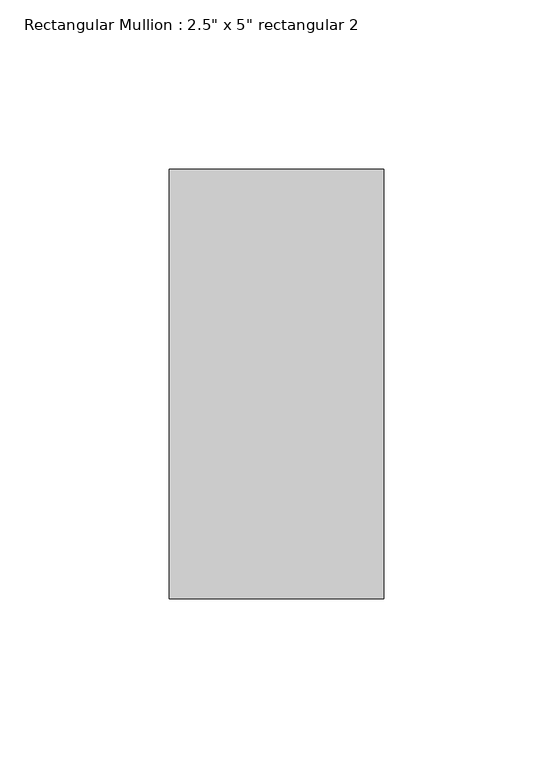
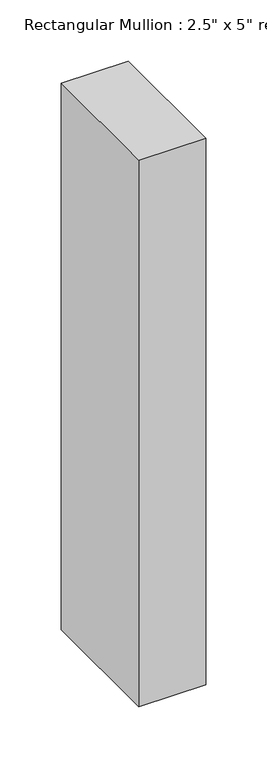
"""IFC4 building model written with IfcOpenShell, lengths in millimetres: member geometry."""

from ifc_helpers import new_model, si_unit, frame, origin, place, context, project, spatial, polyline, outline, extrude, source, transform, mapped, element, save


def member_a980948f(model_context):
    return source(origin(), model_context, "Body", "SweptSolid", [
        extrude(outline(polyline([(0.0, 63.5), (0.0, -63.5), (-63.5, -63.5), (-63.5, 63.5), (0.0, 63.5)])), frame((0.0, 0.0, -546.1), z_axis=(0.0, 0.0, 1.0), x_axis=(1.0, 0.0, 0.0)), (0.0, 0.0, 1.0), 546.1),
    ])


if __name__ == "__main__":
    model = new_model("IFC4")
    model_context = context("Model", 3, world=origin())
    ifc_project = project(units=[si_unit("LENGTHUNIT", "METRE", prefix="MILLI")], contexts=[model_context])
    site = spatial("IfcSite", under=ifc_project)
    building = spatial("IfcBuilding", under=site)
    placement = place(None, origin())
    member_shape = member_a980948f(model_context)
    element("IfcMember", 1, ObjectType="Rectangular Mullion : 2.5\" x 5\" rectangular 2", at=placement, inside=building, context=model_context, shape_type="MappedRepresentation", body=[
        mapped(member_shape, transform((0.0, 0.0, 0.0), x_axis=(1.0, 0.0, 0.0), y_axis=(0.0, 1.0, 0.0), z_axis=(0.0, 0.0, 1.0))),
    ])
    save(model, "model.ifc")

# Revit data of these elements
# Type "Rectangular Mullion : 2.5\" x 5\" rectangular 2"
#   built-in parameter 1007304 = 0.416667 (stored number, unit not read)
#   built-in parameter 1007301 = 0.104167 (stored number, unit not read)
#   built-in parameter 1007300 = 0.104167 (stored number, unit not read)
